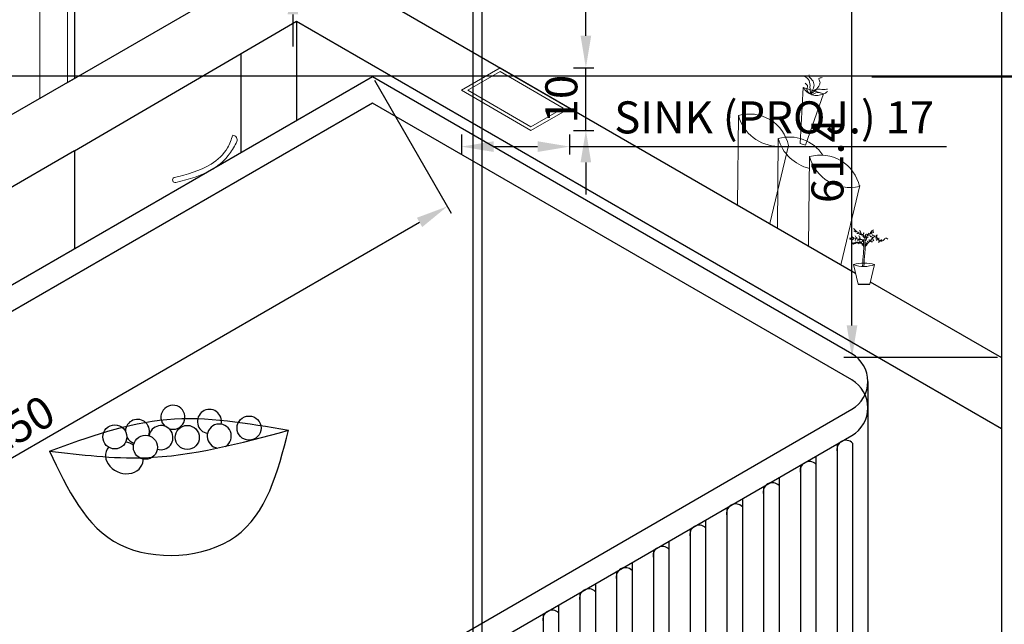
# Model space of a CAD drawing. Units: centimetres. Extents: x 2148 to 2649, y 4226 to 4785.
# Tile 3 of 6: x 2402 to 2555, y 4445 to 4539. Entities that reach past the tile are written whole.
import ezdxf

# ---------------------------------------------------------------- set-up
doc = ezdxf.new("R2010")
doc.units = ezdxf.units.CM
for name, color, linetype, lineweight in [('A-ANNO-DIMS', 63, 'Continuous', 18), ('A-FLOR-BSPL', 21, 'Continuous', 13), ('A-FLOR-CASE', 21, 'Continuous', 25), ('A-FLOR-CASE-HDW', 21, 'Continuous', 18), ('A-FLOR-CASE-TALL', 30, 'Continuous', 30), ('A-FLOR-CTOP', 21, 'Continuous', 25), ('A-FLOR-FIXT', 21, 'Continuous', 18), ('A-FURN-ACCS', 21, 'Continuous', 13), ('TABLE', 30, 'Continuous', 25), ('TREES', 80, 'Continuous', 13)]:
    doc.layers.add(name, color=color, linetype=linetype, lineweight=lineweight)
doc.styles.get("Standard").update_dxf_attribs({"font": 'arial.ttf'})
doc.dimstyles.new('ISO-25', dxfattribs={"dimtxt": 5, "dimasz": 5, "dimexe": 1.25, "dimexo": 0.625, "dimtad": 1, "dimdec": 1, "dimtxsty": 'Standard', "dimcen": 2.5, "dimadec": 0, "dimazin": 0, "dimtfac": 1, "dimtdec": 1, "dimtmove": 0, "dimatfit": 3, "dimfxl": 1, "dimarcsym": 0})

# ---------------------------------------------------------------- blocks, each defined once
blk = doc.blocks.new('RECTANGLE')
for p, q in [((2256.66, 4502.65), (2260.99, 4505.15)), ((2260.99, 4443.76), (2260.99, 4505.15)), ((2256.66, 4502.65), (2256.66, 4441.26)), ((2256.66, 4441.26), (2260.99, 4443.76))]:
    blk.add_line(p, q)
blk = doc.blocks.new('SINK')
for p, q in [((2459.2, 4541.73), (2453.17, 4538.25)), ((2459.2, 4541.73), (2470.05, 4535.47)), ((2459.2, 4541.15), (2454.17, 4538.25)), ((2459.2, 4541.15), (2469.05, 4535.47)), ((2453.17, 4538.25), (2464.01, 4531.98)), ((2454.17, 4538.25), (2464.01, 4532.56)), ((2464.01, 4531.98), (2470.05, 4535.47)), ((2464.01, 4532.56), (2469.05, 4535.47))]:
    blk.add_line(p, q)
blk = doc.blocks.new('TREE')
for p, q in [((2447.25, 4544.96), (2445.48, 4552.43)), ((2451.66, 4544.96), (2453.53, 4552.48))]:
    blk.add_line(p, q)
for centre, radius, start, end in [((2449.6, 4537.88), 15.12, 74.9103, 105.8034), ((2449.44, 4562.68), 11, 248.8663, 291.8473)]:
    blk.add_arc(centre, radius, start, end)
for points, knots in [([(2449.83, 4561.3), (2449.83, 4562.01), (2449.83, 4563.42), (2448.06, 4564.55), (2446.36, 4565.02), (2445.78, 4565.95), (2445.51, 4566.39)], [0, 0, 0, 0, 1.995568, 3.979762, 5.67782, 7.159715, 7.159715, 7.159715, 7.159715]), ([(2445.6, 4565.25), (2445.73, 4565.27), (2445.99, 4565.3), (2446.12, 4564.73), (2446.58, 4565.24), (2446.9, 4564.89), (2447.12, 4564.82), (2447.24, 4564.78)], [0, 0, 0, 0, 0.353698, 0.687974, 1.179754, 1.508828, 1.893119, 1.893119, 1.893119, 1.893119]), ([(2446.1, 4563.4), (2446.2, 4563.04), (2446.31, 4562.66), (2446.75, 4562.63), (2446.69, 4562.48), (2446.67, 4562.4), (2446.66, 4562.35)], [0, 0, 0, 0, 0.953341, 1.006749, 1.098323, 1.293043, 1.293043, 1.293043, 1.293043]), ([(2446.66, 4564.4), (2446.82, 4564.33), (2447.08, 4564.23), (2447.48, 4564.53), (2447.88, 4564.52), (2448.14, 4564.42), (2448.2, 4564.4)], [0, 0, 0, 0, 0.487977, 0.748703, 1.415993, 1.585236, 1.585236, 1.585236, 1.585236]), ([(2447.33, 4563.41), (2447.58, 4563.34), (2447.94, 4563.23), (2447.89, 4562.8), (2447.59, 4562.63), (2448.15, 4562.5), (2448.05, 4562.06), (2448.25, 4562.06), (2448.31, 4562.06)], [0, 0, 0, 0, 0.664801, 0.94436, 1.08206, 1.476917, 1.846316, 2.003009, 2.003009, 2.003009, 2.003009]), ([(2447.76, 4563.97), (2447.97, 4563.94), (2448.19, 4563.91), (2448.52, 4563.93), (2448.62, 4563.77), (2448.92, 4563.75), (2449.11, 4563.68), (2449.26, 4563.62)], [0, 0, 0, 0, 0.637067, 0.675943, 0.960411, 1.092541, 1.560471, 1.560471, 1.560471, 1.560471]), ([(2447.89, 4565.62), (2447.89, 4565.43), (2447.89, 4565.1), (2448.34, 4564.81), (2448.24, 4564.52), (2448.19, 4564.38)], [0, 0, 0, 0, 0.528266, 0.942976, 1.342243, 1.342243, 1.342243, 1.342243]), ([(2448.99, 4563.3), (2449.11, 4563.19), (2449.28, 4563.05), (2449.5, 4562.84), (2449.63, 4562.83), (2449.7, 4562.83)], [0, 0, 0, 0, 0.4862835, 0.6806136, 0.871086, 0.871086, 0.871086, 0.871086]), ([(2449.26, 4563.62), (2449.19, 4563.84), (2449.08, 4564.17), (2449.43, 4564.46), (2449.34, 4564.59), (2449.31, 4564.63)], [0, 0, 0, 0, 0.636403, 0.920765, 1.065556, 1.065556, 1.065556, 1.065556]), ([(2450.14, 4564.1), (2450.1, 4563.96), (2450, 4563.68), (2450.06, 4563.32), (2449.98, 4562.88), (2449.68, 4562.82), (2449.46, 4562.77)], [0, 0, 0, 0, 0.427172, 0.880416, 1.093996, 1.685063, 1.685063, 1.685063, 1.685063]), ([(2449.83, 4561.3), (2450.13, 4561.73), (2450.64, 4562.45), (2450.53, 4563.72), (2451.5, 4564.19), (2452.37, 4564.56), (2452.66, 4565.2), (2452.78, 4565.47)], [0, 0, 0, 0, 1.559218, 2.590263, 3.316916, 4.501885, 5.353772, 5.353772, 5.353772, 5.353772]), ([(2449.98, 4559.44), (2450.53, 4560.09), (2451.61, 4561.35), (2454.23, 4564.3), (2454.67, 4561.58), (2456.89, 4561.05), (2457.55, 4562.97), (2458.29, 4562.41), (2458.61, 4562.17)], [0, 0, 0, 0, 2.950259, 5.736815, 7.202351, 9.196187, 10.495572, 11.481506, 11.481506, 11.481506, 11.481506]), ([(2450.65, 4563.53), (2450.67, 4563.63), (2450.7, 4563.82), (2450.57, 4564.03), (2450.57, 4564.16), (2450.57, 4564.2)], [0, 0, 0, 0, 0.2987758, 0.5629986, 0.6917618, 0.6917618, 0.6917618, 0.6917618]), ([(2450.79, 4563.5), (2450.85, 4563.54), (2451.15, 4563.74), (2451.53, 4563.69), (2451.84, 4563.65)], [0, 0, 0, 0, 0.18742, 1.072841, 1.072841, 1.072841, 1.072841]), ([(2451.14, 4564.01), (2451.19, 4564.03), (2451.33, 4564.07), (2451.2, 4564.29), (2451.26, 4564.44), (2451.3, 4564.5), (2451.32, 4564.51)], [0, 0, 0, 0, 0.131224, 0.3928497, 0.5275017, 0.5966013, 0.5966013, 0.5966013, 0.5966013]), ([(2451.65, 4564.25), (2451.78, 4564.27), (2452.08, 4564.3), (2452.39, 4564.26), (2452.56, 4564.23)], [0, 0, 0, 0, 0.388997, 0.9136239, 0.9136239, 0.9136239, 0.9136239]), ([(2452.65, 4562.49), (2452.63, 4562.64), (2452.59, 4562.93), (2452.3, 4563.47), (2451.98, 4563.24), (2451.82, 4563.12)], [0, 0, 0, 0, 0.45479, 0.92627, 1.425708, 1.425708, 1.425708, 1.425708]), ([(2451.9, 4564.38), (2451.95, 4564.49), (2452.04, 4564.65), (2452.01, 4564.87), (2452.01, 4564.97), (2452.01, 4565)], [0, 0, 0, 0, 0.3358398, 0.5448262, 0.633178, 0.633178, 0.633178, 0.633178]), ([(2452.27, 4564.64), (2452.32, 4564.72), (2452.48, 4564.99), (2452.99, 4564.61), (2453.14, 4564.98), (2453.12, 4565.11), (2453.12, 4565.16)], [0, 0, 0, 0, 0.251714, 0.837833, 1.078551, 1.22335, 1.22335, 1.22335, 1.22335]), ([(2452.4, 4564.8), (2452.41, 4564.88), (2452.43, 4565.06), (2452.32, 4565.32), (2452.44, 4565.42), (2452.47, 4565.45)], [0, 0, 0, 0, 0.2491213, 0.5552893, 0.6860823, 0.6860823, 0.6860823, 0.6860823]), ([(2452.72, 4565.33), (2452.73, 4565.38), (2452.79, 4565.56), (2453.08, 4565.6), (2453.11, 4565.76), (2453.12, 4565.78)], [0, 0, 0, 0, 0.1482784, 0.5567745, 0.6230075, 0.6230075, 0.6230075, 0.6230075]), ([(2453.57, 4563.27), (2453.54, 4563.35), (2453.44, 4563.57), (2453.12, 4563.6), (2452.91, 4563.7), (2452.68, 4563.58), (2452.8, 4563.73), (2452.87, 4563.82)], [0, 0, 0, 0, 0.250514, 0.700182, 0.817059, 0.973893, 1.195588, 1.195588, 1.195588, 1.195588]), ([(2454.21, 4563.26), (2454.25, 4563.33), (2454.32, 4563.45), (2454.32, 4563.75), (2454.55, 4563.67), (2454.65, 4563.66), (2454.69, 4563.66)], [0, 0, 0, 0, 0.2405941, 0.4530054, 0.6562483, 0.7710751, 0.7710751, 0.7710751, 0.7710751]), ([(2449.39, 4560.41), (2449.32, 4560.98), (2449.16, 4562.11), (2447.09, 4562.07), (2445.55, 4562.82), (2444.32, 4562.59), (2443.85, 4562.5)], [0, 0, 0, 0, 1.50196, 2.979977, 5.268293, 6.6547, 6.6547, 6.6547, 6.6547]), ([(2444.83, 4562.66), (2444.5, 4562.55), (2444.06, 4562.4), (2444.1, 4562), (2444.11, 4561.9)], [0, 0, 0, 0, 0.86957, 1.154464, 1.154464, 1.154464, 1.154464]), ([(2444.53, 4563.19), (2444.82, 4563.13), (2445.18, 4563.05), (2445.34, 4562.62), (2445.49, 4562.62), (2445.55, 4562.62)], [0, 0, 0, 0, 0.799643, 1.030684, 1.19755, 1.19755, 1.19755, 1.19755]), ([(2449.45, 4559.33), (2448.92, 4560.14), (2448.1, 4561.4), (2446.22, 4560.44), (2445.17, 4560.51), (2444.56, 4560.54)], [0, 0, 0, 0, 2.40992, 3.739305, 5.578847, 5.578847, 5.578847, 5.578847]), ([(2445.01, 4560.71), (2445.17, 4560.62), (2445.37, 4560.5), (2445.62, 4560.51), (2445.68, 4560.52), (2445.69, 4560.52)], [0, 0, 0, 0, 0.5295015, 0.6942572, 0.7168035, 0.7168035, 0.7168035, 0.7168035]), ([(2445.55, 4562.62), (2445.49, 4562.52), (2445.4, 4562.36), (2445.26, 4562.12), (2445.18, 4561.91), (2445.06, 4561.89), (2445.04, 4561.89)], [0, 0, 0, 0, 0.3536471, 0.5448852, 0.8584322, 0.9118713, 0.9118713, 0.9118713, 0.9118713]), ([(2445.19, 4560.23), (2445.23, 4560.26), (2445.34, 4560.32), (2445.53, 4560.36), (2445.62, 4560.47), (2445.66, 4560.52)], [0, 0, 0, 0, 0.157145, 0.3589113, 0.5662429, 0.5662429, 0.5662429, 0.5662429]), ([(2445.61, 4560.86), (2445.67, 4560.79), (2445.79, 4560.65), (2445.97, 4560.57), (2446.2, 4560.56), (2446.18, 4560.62), (2446.18, 4560.64)], [0, 0, 0, 0, 0.2483933, 0.5604364, 0.6736581, 0.7258462, 0.7258462, 0.7258462, 0.7258462]), ([(2446.61, 4562.36), (2446.46, 4562.28), (2446.22, 4562.17), (2446.12, 4561.86), (2446.12, 4561.72), (2446.13, 4561.68)], [0, 0, 0, 0, 0.4813649, 0.7680471, 0.8975493, 0.8975493, 0.8975493, 0.8975493]), ([(2446.22, 4561.18), (2446.38, 4560.89), (2446.62, 4560.47), (2446.85, 4561.06), (2447.05, 4560.94), (2447.15, 4560.88)], [0, 0, 0, 0, 0.64318, 0.967785, 1.239353, 1.239353, 1.239353, 1.239353]), ([(2448.31, 4562.06), (2448.14, 4561.91), (2447.81, 4561.63), (2447.17, 4562.12), (2447.11, 4561.73), (2447.09, 4561.57)], [0, 0, 0, 0, 0.622646, 1.172708, 1.557766, 1.557766, 1.557766, 1.557766]), ([(2447.66, 4560.97), (2447.54, 4560.94), (2447.32, 4560.88), (2447.34, 4560.55), (2447.21, 4560.45), (2447.15, 4560.41)], [0, 0, 0, 0, 0.333136, 0.6124023, 0.8146283, 0.8146283, 0.8146283, 0.8146283]), ([(2447.69, 4560.54), (2447.73, 4560.56), (2447.88, 4560.64), (2448.15, 4560.5), (2448.26, 4560.67), (2448.31, 4560.74)], [0, 0, 0, 0, 0.1577786, 0.4768013, 0.6980293, 0.6980293, 0.6980293, 0.6980293]), ([(2447.73, 4561.36), (2447.81, 4561.27), (2447.9, 4561.16), (2448.03, 4561), (2448.13, 4560.92), (2448.11, 4560.85), (2448.11, 4560.84)], [0, 0, 0, 0, 0.3534347, 0.4287436, 0.6404395, 0.6555943, 0.6555943, 0.6555943, 0.6555943]), ([(2448.68, 4560.4), (2448.6, 4560.54), (2448.48, 4560.74), (2448.57, 4561.03), (2448.51, 4561.14), (2448.48, 4561.19)], [0, 0, 0, 0, 0.4503193, 0.6632194, 0.8315566, 0.8315566, 0.8315566, 0.8315566]), ([(2448.59, 4560), (2448.64, 4560.01), (2448.72, 4560.02), (2448.85, 4559.94), (2448.99, 4559.99), (2449.05, 4559.93), (2449.05, 4559.93)], [0, 0, 0, 0, 0.1309766, 0.2265734, 0.4607298, 0.4703086, 0.4703086, 0.4703086, 0.4703086]), ([(2449.25, 4561.22), (2449.08, 4561.38), (2448.82, 4561.62), (2448.7, 4561.25), (2448.74, 4561.15), (2448.74, 4561.13)], [0, 0, 0, 0, 0.4936671, 0.7765002, 0.8174683, 0.8174683, 0.8174683, 0.8174683]), ([(2448.91, 4551.67), (2449, 4553.4), (2449.11, 4555.46), (2449.34, 4558.06), (2449.53, 4559.55), (2449.32, 4560.95), (2449.26, 4561.81), (2449.24, 4562.05)], [0, 0, 0, 0, 5.198408, 6.198659, 7.833196, 9.680738, 10.407711, 10.407711, 10.407711, 10.407711]), ([(2449.05, 4559.93), (2449.07, 4560.03), (2449.1, 4560.2), (2449.14, 4560.46), (2449.08, 4560.61), (2449.04, 4560.7)], [0, 0, 0, 0, 0.3315498, 0.4956558, 0.7928621, 0.7928621, 0.7928621, 0.7928621]), ([(2449.44, 4551.69), (2449.53, 4553.42), (2449.64, 4555.48), (2449.87, 4558.08), (2450.05, 4559.57), (2449.85, 4560.97), (2449.78, 4561.83), (2449.77, 4562.07)], [0, 0, 0, 0, 5.198408, 6.198659, 7.833196, 9.680738, 10.407711, 10.407711, 10.407711, 10.407711]), ([(2450.35, 4559.88), (2450.3, 4560.05), (2450.24, 4560.27), (2450.53, 4560.53), (2450.4, 4560.73), (2450.3, 4560.87)], [0, 0, 0, 0, 0.457334, 0.622454, 1.040097, 1.040097, 1.040097, 1.040097]), ([(2450.36, 4562.16), (2450.35, 4562.24), (2450.34, 4562.38), (2450.26, 4562.64), (2450.36, 4562.81), (2450.42, 4562.91)], [0, 0, 0, 0, 0.2419015, 0.4294094, 0.782934, 0.782934, 0.782934, 0.782934]), ([(2450.53, 4562.68), (2450.57, 4562.72), (2450.64, 4562.77), (2450.72, 4562.83), (2450.82, 4562.94), (2451.03, 4562.88), (2451.1, 4563), (2451.12, 4563.03)], [0, 0, 0, 0, 0.1839825, 0.2354423, 0.32084, 0.6015787, 0.715757, 0.715757, 0.715757, 0.715757]), ([(2451.04, 4560.68), (2451.04, 4560.78), (2451.05, 4560.99), (2450.8, 4561.22), (2450.91, 4561.38), (2450.96, 4561.45)], [0, 0, 0, 0, 0.308616, 0.5966018, 0.8330049, 0.8330049, 0.8330049, 0.8330049]), ([(2451.4, 4561.1), (2452.09, 4561.38), (2452.96, 4561.74), (2452.35, 4561.06), (2452.51, 4561), (2452.56, 4560.99)], [0, 0, 0, 0, 1.194027, 1.500255, 1.630788, 1.630788, 1.630788, 1.630788]), ([(2451.48, 4561.19), (2451.51, 4561.32), (2451.55, 4561.5), (2451.46, 4561.77), (2451.47, 4561.92), (2451.48, 4562.03)], [0, 0, 0, 0, 0.3935209, 0.5296667, 0.851575, 0.851575, 0.851575, 0.851575]), ([(2452.32, 4562.14), (2452.6, 4562.23), (2453.1, 4562.38), (2452.98, 4561.72), (2453.18, 4561.6), (2453.24, 4561.57)], [0, 0, 0, 0, 0.657659, 1.152477, 1.342596, 1.342596, 1.342596, 1.342596]), ([(2454.41, 4562.99), (2454.17, 4562.89), (2453.74, 4562.72), (2454.23, 4562.34), (2454.12, 4562.17), (2454.1, 4562.14)], [0, 0, 0, 0, 0.56032, 1.008165, 1.121509, 1.121509, 1.121509, 1.121509]), ([(2454.61, 4562.45), (2454.46, 4562.3), (2454.24, 4562.09), (2454.49, 4561.73), (2454.33, 4561.66), (2454.26, 4561.63)], [0, 0, 0, 0, 0.537826, 0.7745438, 0.9749671, 0.9749671, 0.9749671, 0.9749671]), ([(2455.47, 4561.55), (2455.41, 4561.46), (2455.3, 4561.31), (2455.4, 4560.89), (2455.07, 4560.99), (2454.85, 4561.05)], [0, 0, 0, 0, 0.329722, 0.545126, 1.027082, 1.027082, 1.027082, 1.027082]), ([(2454.99, 4561.88), (2455.08, 4561.98), (2455.24, 4562.14), (2455.11, 4562.39), (2455.18, 4562.62), (2455.26, 4562.61), (2455.28, 4562.61)], [0, 0, 0, 0, 0.3499692, 0.6062162, 0.8045661, 0.8552851, 0.8552851, 0.8552851, 0.8552851]), ([(2455.86, 4561.43), (2455.78, 4561.56), (2455.6, 4561.89), (2456.32, 4561.69), (2456.26, 4561.99), (2456.23, 4562.1)], [0, 0, 0, 0, 0.333961, 0.823844, 1.08993, 1.08993, 1.08993, 1.08993])]:
    blk.add_open_spline(points, degree=3, knots=knots)
blk = doc.blocks.new('T')
for p, q in [((2448.14, 4353.09), (2318.24, 4278.09)), ((2522.91, 4309.92), (2448.14, 4353.09)), ((2403.01, 4232.03), (2522.91, 4301.26))]:
    blk.add_line(p, q)
blk.add_arc((2520.41, 4305.59), 5, 300, 60)
blk = doc.blocks.new('FRUITS')
for centre in [(2437.55, 4475.46), (2416.61, 4474.09), (2427.91, 4474), (2421.39, 4472.47)]:
    blk.add_circle(centre, 1.88)
for centre, start, end in [((2425.68, 4477.15), 250.6785, 228.1131), ((2431.37, 4476.49), 347.1742, 260.6235), ((2420.14, 4474.94), 339.5983, 177.9649), ((2423.8, 4473.97), 252.9307, 170.9248), ((2432.9, 4474.21), 301.9934, 262.6603), ((2420.14, 4474.94), 208.8656, 254.0869)]:
    blk.add_arc(centre, 1.88, start, end)
for start_param, end_param in [(4.471607, 4.914134), (5.976427, 9.8373)]:
    blk.add_ellipse((2418.08, 4470.84), major_axis=(-2.82, 1), ratio=0.809593, start_param=start_param, end_param=end_param)
for points, knots in [([(2406.43, 4471.88), (2412.49, 4474.08), (2424.62, 4478.48), (2437.33, 4476.24), (2443.7, 4475.12)], [0, 0, 0, 0, 18.967698, 37.99902, 37.99902, 37.99902, 37.99902]), ([(2406.43, 4471.88), (2409.22, 4465.94), (2414.78, 4454.12), (2438.7, 4455.69), (2442.02, 4468.59), (2443.7, 4475.12)], [0, 0, 0, 0, 18.249558, 36.298645, 54.808813, 54.808813, 54.808813, 54.808813]), ([(2406.43, 4471.88), (2411.36, 4471.29), (2423.93, 4469.77), (2436.23, 4473.1), (2443.7, 4475.12)], [0, 0, 0, 0, 14.783083, 37.710843, 37.710843, 37.710843, 37.710843])]:
    blk.add_open_spline(points, degree=3, knots=knots)
blk = doc.blocks.new('TABLE 3')
for p, q in [((2534.09, 4482.72), (2534.09, 4425.1)), ((2529.29, 4472.97), (2529.29, 4424.6)), ((2531.69, 4473.13), (2531.69, 4424.8)), ((2531.69, 4473.13), (2531.69, 4424.8)), ((2525.96, 4471.05), (2525.96, 4423.89)), ((2529.29, 4471.74), (2529.29, 4424.6)), ((2523.55, 4469.66), (2523.55, 4424.61)), ((2525.96, 4469.82), (2525.96, 4423.89)), ((2523.55, 4468.43), (2523.55, 4424.61)), ((2520.23, 4467.74), (2520.23, 4430.04)), ((2520.23, 4466.51), (2520.23, 4430.04)), ((2517.82, 4466.35), (2517.82, 4432.4)), ((2517.82, 4465.12), (2517.82, 4432.4)), ((2514.5, 4464.43), (2514.5, 4434.64)), ((2512.09, 4463.04), (2512.09, 4434.39)), ((2512.09, 4461.81), (2512.09, 4434.39)), ((2514.5, 4463.2), (2514.5, 4434.64)), ((2508.76, 4461.12), (2508.76, 4432.32)), ((2506.35, 4459.73), (2506.35, 4430.48)), ((2503.03, 4457.81), (2503.03, 4427.36)), ((2506.35, 4458.5), (2506.35, 4430.48)), ((2500.62, 4456.42), (2500.62, 4424.52)), ((2503.03, 4456.58), (2503.03, 4427.36)), ((2497.3, 4454.5), (2497.3, 4419.33)), ((2500.62, 4455.19), (2500.62, 4424.52)), ((2494.89, 4453.11), (2494.89, 4413.65)), ((2497.3, 4453.27), (2497.3, 4419.33)), ((2491.57, 4451.19), (2491.57, 4413.39)), ((2494.89, 4451.88), (2494.89, 4413.65)), ((2489.16, 4449.8), (2489.16, 4412.9)), ((2491.57, 4449.96), (2491.57, 4413.39)), ((2489.16, 4448.57), (2489.16, 4412.9)), ((2483.42, 4446.49), (2483.42, 4412.26)), ((2485.83, 4447.88), (2485.83, 4412.44)), ((2485.83, 4446.65), (2485.83, 4412.44)), ((2483.42, 4445.26), (2483.42, 4412.26))]:
    blk.add_line(p, q)
for centre in [(2530.67, 4472.12), (2524.94, 4468.81), (2519.2, 4465.5), (2513.47, 4462.19), (2507.74, 4458.88), (2502.01, 4455.57), (2496.27, 4452.26), (2490.54, 4448.95), (2484.81, 4445.64)]:
    blk.add_arc(centre, 1.44, 44.5272, 195.4728)
for name, p in [('T', (8.67, 177.13)), ('T', (8.67, 173.04)), ('FRUITS', (0, 0))]:
    blk.add_blockref(name, p)
blk = doc.blocks.new('PULL-BASE-BOW')
for centre, radius, start, end in [((9.29, 6.64), 0.774, 341.702, 83.222), ((0.41, 0.41), 0.414, 116.0189, 282.6641)]:
    blk.add_arc(centre, radius, start, end)
for points, knots in [([(0.23, 0.79), (2.23, 1.29), (5.42, 2.1), (8.53, 4.9), (9.15, 6.73), (9.38, 7.41)], [0, 0, 0, 0, 6.127515, 9.756066, 11.887711, 11.887711, 11.887711, 11.887711]), ([(0.5, 0.01), (2.55, 0.54), (5.72, 1.35), (8.78, 4.08), (9.68, 5.75), (10.03, 6.4)], [0, 0, 0, 0, 6.234589, 9.67204, 11.894402, 11.894402, 11.894402, 11.894402])]:
    blk.add_open_spline(points, degree=3, knots=knots)
blk = doc.blocks.new('*D28')
at = {"layer": 'A-ANNO-DIMS', "color": 0, "lineweight": -2, "transparency": 16777216}
for p, q in [((2470.68, 4521.25), (2470.68, 4518.09)), ((2487.56, 4521.25), (2487.56, 4518.09)), ((2475.68, 4519.34), (2482.56, 4519.34)), ((2487.56, 4519.34), (2546.35, 4519.34))]:
    blk.add_line(p, q, dxfattribs=at)
at = {"layer": 'A-ANNO-DIMS', "color": 0, "transparency": 16777216}
for points in [[(2475.68, 4520.17), (2475.68, 4518.51), (2470.68, 4519.34)], [(2482.56, 4520.17), (2482.56, 4518.51), (2487.56, 4519.34)]]:
    blk.add_solid(points, dxfattribs=at)
at = {"layer": 'Defpoints', "color": 0, "transparency": 16777216}
for p in [(2470.68, 4521.87), (2487.56, 4521.87), (2487.56, 4519.34)]:
    blk.add_point(p, dxfattribs=at)
at = {"layer": 'A-ANNO-DIMS', "color": 0, "transparency": 16777216, "insert": (2519.46, 4523.25), "char_height": 5, "attachment_point": 5}
blk.add_mtext('SINK (PROJ.) 17', dxfattribs=at)
blk = doc.blocks.new('*D29')
at = {"layer": 'A-ANNO-DIMS', "color": 0, "lineweight": -2, "transparency": 16777216}
for p, q in [((2490.09, 4536.62), (2490.09, 4541.62)), ((2488.18, 4531.62), (2491.34, 4531.62)), ((2490.09, 4521.87), (2490.09, 4531.62)), ((2488.18, 4521.87), (2491.34, 4521.87)), ((2490.09, 4516.87), (2490.09, 4511.87))]:
    blk.add_line(p, q, dxfattribs=at)
at = {"layer": 'A-ANNO-DIMS', "color": 0, "transparency": 16777216}
for points in [[(2489.26, 4536.62), (2490.92, 4536.62), (2490.09, 4531.62)], [(2489.26, 4516.87), (2490.92, 4516.87), (2490.09, 4521.87)]]:
    blk.add_solid(points, dxfattribs=at)
at = {"layer": 'Defpoints', "color": 0, "transparency": 16777216}
for p in [(2487.56, 4531.62), (2490.09, 4531.62), (2487.56, 4521.87)]:
    blk.add_point(p, dxfattribs=at)
at = {"layer": 'A-ANNO-DIMS', "color": 0, "transparency": 16777216, "insert": (2486.91, 4526.75), "char_height": 5, "attachment_point": 5, "rotation": 90}
blk.add_mtext('10', dxfattribs=at)
blk = doc.blocks.new('*D30')
at = {"layer": 'A-ANNO-DIMS', "color": 0, "lineweight": -2, "transparency": 16777216}
for p, q in [((2534.71, 4530.22), (2574.8, 4530.22)), ((2573.55, 4272.15), (2573.55, 4525.22)), ((2534.71, 4267.15), (2574.8, 4267.15))]:
    blk.add_line(p, q, dxfattribs=at)
at = {"layer": 'A-ANNO-DIMS', "color": 0, "transparency": 16777216}
for points in [[(2572.71, 4525.22), (2574.38, 4525.22), (2573.55, 4530.22)], [(2572.71, 4272.15), (2574.38, 4272.15), (2573.55, 4267.15)]]:
    blk.add_solid(points, dxfattribs=at)
at = {"layer": 'Defpoints', "color": 0, "transparency": 16777216}
for p in [(2534.09, 4530.22), (2573.55, 4530.22), (2534.09, 4267.15)]:
    blk.add_point(p, dxfattribs=at)
at = {"layer": 'A-ANNO-DIMS', "color": 0, "transparency": 16777216, "insert": (2569.64, 4398.69), "char_height": 5, "attachment_point": 5, "rotation": 90}
blk.add_mtext('ISLAND (PROJ.) 263', dxfattribs=at)
blk = doc.blocks.new('*D38')
at = {"layer": 'A-ANNO-DIMS', "color": 0, "lineweight": -2, "transparency": 16777216}
for p, q in [((2444.39, 4558.67), (2444.39, 4609.58)), ((2443.71, 4553.67), (2445.64, 4553.67)), ((2444.39, 4544.96), (2444.39, 4553.67)), ((2443.71, 4544.96), (2445.64, 4544.96)), ((2444.39, 4539.96), (2444.39, 4534.96))]:
    blk.add_line(p, q, dxfattribs=at)
at = {"layer": 'A-ANNO-DIMS', "color": 0, "transparency": 16777216}
for points in [[(2443.56, 4558.67), (2445.22, 4558.67), (2444.39, 4553.67)], [(2443.56, 4539.96), (2445.22, 4539.96), (2444.39, 4544.96)]]:
    blk.add_solid(points, dxfattribs=at)
at = {"layer": 'Defpoints', "color": 0, "transparency": 16777216}
for p in [(2443.09, 4553.67), (2444.39, 4553.67), (2443.09, 4544.96)]:
    blk.add_point(p, dxfattribs=at)
at = {"layer": 'A-ANNO-DIMS', "color": 0, "transparency": 16777216, "insert": (2441.21, 4586.62), "char_height": 5, "attachment_point": 5, "rotation": 90}
blk.add_mtext('PLANT 9 TYP.', dxfattribs=at)
blk = doc.blocks.new('*D44')
at = {"layer": 'A-ANNO-DIMS', "color": 0, "lineweight": -2, "transparency": 16777216}
for p, q in [((2305.27, 4564.32), (2648.78, 4564.32)), ((2647.53, 4559.32), (2647.53, 4535.36)), ((2305.27, 4530.36), (2648.78, 4530.36))]:
    blk.add_line(p, q, dxfattribs=at)
at = {"layer": 'A-ANNO-DIMS', "color": 0, "transparency": 16777216}
for points in [[(2646.7, 4559.32), (2648.37, 4559.32), (2647.53, 4564.32)], [(2646.7, 4535.36), (2648.37, 4535.36), (2647.53, 4530.36)]]:
    blk.add_solid(points, dxfattribs=at)
at = {"layer": 'Defpoints', "color": 0, "transparency": 16777216}
for p in [(2304.65, 4564.32), (2304.65, 4530.36), (2647.53, 4530.36)]:
    blk.add_point(p, dxfattribs=at)
at = {"layer": 'A-ANNO-DIMS', "color": 0, "transparency": 16777216, "insert": (2644.35, 4547.34), "char_height": 5, "attachment_point": 5, "rotation": 90}
blk.add_mtext('33.96', dxfattribs=at)
blk = doc.blocks.new('*D48')
at = {"layer": 'A-ANNO-DIMS', "color": 0, "lineweight": -2, "transparency": 16777216}
for p, q in [((2472.44, 4594.86), (2472.44, 4242.8)), ((2473.86, 4594.94), (2473.86, 4242.8)), ((2467.44, 4244.05), (2462.44, 4244.05)), ((2472.44, 4244.05), (2473.86, 4244.05)), ((2478.86, 4244.05), (2497.57, 4244.05))]:
    blk.add_line(p, q, dxfattribs=at)
at = {"layer": 'A-ANNO-DIMS', "color": 0, "transparency": 16777216}
for points in [[(2467.44, 4244.88), (2467.44, 4243.21), (2472.44, 4244.05)], [(2478.86, 4244.88), (2478.86, 4243.21), (2473.86, 4244.05)]]:
    blk.add_solid(points, dxfattribs=at)
at = {"layer": 'Defpoints', "color": 0, "transparency": 16777216}
for p in [(2472.44, 4595.48), (2473.86, 4595.56), (2473.86, 4244.05)]:
    blk.add_point(p, dxfattribs=at)
at = {"layer": 'A-ANNO-DIMS', "color": 0, "transparency": 16777216, "insert": (2490.71, 4247.18), "char_height": 5, "attachment_point": 5}
blk.add_mtext('1.42', dxfattribs=at)
blk = doc.blocks.new('*D51')
at = {"layer": 'A-ANNO-DIMS', "color": 0, "lineweight": -2, "transparency": 16777216}
for p, q in [((2436.91, 4714.24), (2648.78, 4714.24)), ((2647.53, 4272.37), (2647.53, 4709.24)), ((2409.81, 4267.37), (2648.78, 4267.37))]:
    blk.add_line(p, q, dxfattribs=at)
at = {"layer": 'A-ANNO-DIMS', "color": 0, "transparency": 16777216}
for points in [[(2646.7, 4709.24), (2648.37, 4709.24), (2647.53, 4714.24)], [(2646.7, 4272.37), (2648.37, 4272.37), (2647.53, 4267.37)]]:
    blk.add_solid(points, dxfattribs=at)
at = {"layer": 'Defpoints', "color": 0, "transparency": 16777216}
for p in [(2436.28, 4714.24), (2647.53, 4714.24), (2409.18, 4267.37)]:
    blk.add_point(p, dxfattribs=at)
at = {"layer": 'A-ANNO-DIMS', "color": 0, "transparency": 16777216, "insert": (2644.36, 4490.81), "char_height": 5, "attachment_point": 5, "rotation": 90}
blk.add_mtext('446.9', dxfattribs=at)
blk = doc.blocks.new('*D58')
at = {"layer": 'A-ANNO-DIMS', "color": 0, "lineweight": -2, "transparency": 16777216}
for p, q in [((2457.13, 4529.68), (2469.1, 4508.94)), ((2464.15, 4507.52), (2342.9, 4437.52)), ((2327.22, 4454.68), (2339.2, 4433.94))]:
    blk.add_line(p, q, dxfattribs=at)
at = {"layer": 'A-ANNO-DIMS', "color": 0, "transparency": 16777216}
for points in [[(2463.73, 4508.25), (2464.56, 4506.8), (2468.48, 4510.02)], [(2342.49, 4438.25), (2343.32, 4436.8), (2338.57, 4435.02)]]:
    blk.add_solid(points, dxfattribs=at)
at = {"layer": 'Defpoints', "color": 0, "transparency": 16777216}
for p in [(2456.81, 4530.22), (2326.91, 4455.22), (2338.57, 4435.02)]:
    blk.add_point(p, dxfattribs=at)
at = {"layer": 'A-ANNO-DIMS', "color": 0, "transparency": 16777216, "insert": (2401.94, 4475.28), "char_height": 5, "attachment_point": 5, "rotation": 30}
blk.add_mtext('150', dxfattribs=at)
blk = doc.blocks.new('*D59')
at = {"layer": 'A-ANNO-DIMS', "color": 0, "lineweight": -2, "transparency": 16777216}
for p, q in [((2554.3, 4547.86), (2530.35, 4547.86)), ((2531.6, 4491.46), (2531.6, 4542.86)), ((2554.3, 4486.46), (2530.35, 4486.46))]:
    blk.add_line(p, q, dxfattribs=at)
at = {"layer": 'A-ANNO-DIMS', "color": 0, "transparency": 16777216}
for points in [[(2530.77, 4542.86), (2532.43, 4542.86), (2531.6, 4547.86)], [(2530.77, 4491.46), (2532.43, 4491.46), (2531.6, 4486.46)]]:
    blk.add_solid(points, dxfattribs=at)
at = {"layer": 'Defpoints', "color": 0, "transparency": 16777216}
for p in [(2531.6, 4547.86), (2554.93, 4547.86), (2554.93, 4486.46)]:
    blk.add_point(p, dxfattribs=at)
at = {"layer": 'A-ANNO-DIMS', "color": 0, "transparency": 16777216, "insert": (2528.42, 4517.16), "char_height": 5, "attachment_point": 5, "rotation": 90}
blk.add_mtext('61.4', dxfattribs=at)

msp = doc.modelspace()

# ---------------------------------------------------------------- linework, layer by layer
at = {"layer": 'A-FLOR-CASE'}
for p, q in [((2410.3004, 4699.2447), (2410.3004, 4529.9623)), ((2444.9414, 4538.8707), (2444.9414, 4523.3687)), ((2436.2812, 4533.8172), (2436.2812, 4518.3687)), ((2410.3004, 4518.6569), (2410.3004, 4503.3687))]:
    msp.add_line(p, q, dxfattribs=at)
at = {"layer": 'A-FLOR-CASE-TALL'}
msp.add_line((2554.9266, 4645.7447), (2554.9266, 4369.7671), dxfattribs=at)
at = {"layer": 'A-FLOR-CTOP'}
for p, q in [((2409.2302, 4529.3444), (2436.2812, 4544.9623)), ((2453.6017, 4544.9623), (2532.1733, 4499.5989)), ((2410.3004, 4518.6569), (2444.9414, 4538.8707)), ((2444.9414, 4538.8707), (2554.9266, 4475.3707)), ((2410.3004, 4529.9623), (2254.4158, 4439.9623)), ((2410.3004, 4518.6569), (2254.4158, 4428.6569)), ((2532.5706, 4497.9209), (2534.3632, 4497.9209)), ((2534.4534, 4498.2825), (2554.9266, 4486.4623))]:
    msp.add_line(p, q, dxfattribs=at)
at = {"layer": 'A-FURN-ACCS'}
for p, q in [((2513.7427, 4510.2398), (2513.8843, 4524.1808)), ((2519.9592, 4506.6507), (2520.1007, 4520.5917)), ((2521.6845, 4519.5131), (2518.7703, 4507.3371)), ((2524.8302, 4503.8385), (2524.9717, 4517.7794)), ((2532.8065, 4513.256), (2529.8577, 4500.9358)), ((2513.7427, 4510.2398), (2518.7703, 4507.3371)), ((2519.9592, 4506.6507), (2524.9867, 4503.7481)), ((2524.8302, 4503.8385), (2529.8577, 4500.9358))]:
    msp.add_line(p, q, dxfattribs=at)
for centre, radius, start, end in [((2515.6078, 4518.2096), 6.2149, 12.106803, 106.100627), ((2520.2607, 4525.9851), 6.6267, 195.799765, 268.508977), ((2521.8243, 4514.6206), 6.2149, 33.095394, 106.100627), ((2526.4771, 4522.396), 6.6267, 195.799765, 256.704649), ((2526.6953, 4511.8083), 6.2149, 12.106803, 106.100627), ((2531.3481, 4519.5837), 6.6267, 195.799765, 282.407665)]:
    msp.add_arc(centre, radius, start, end, dxfattribs=at)
at = {"layer": 'TABLE'}
msp.add_line((2508.7637, 4459.8889), (2508.7637, 4432.3196), dxfattribs=at)
at = {"layer": 'TREES'}
for p, q in [((2523.5086, 4519.8148), (2524.0096, 4528.579)), ((2524.0096, 4528.579), (2527.1342, 4527.5826)), ((2527.1342, 4527.5826), (2524.3631, 4519.5409)), ((2524.3631, 4519.5409), (2523.5086, 4519.8148))]:
    msp.add_line(p, q, dxfattribs=at)
msp.add_arc((2526.0501, 4529.5804), 2.273, 206.140299, 298.485133, dxfattribs=at)
for points, knots in [([(2525.1443, 4527.5393), (2525.0928, 4527.8926), (2525.0162, 4528.4173), (2525.0929, 4529.2921), (2524.7724, 4529.9979), (2524.3149, 4530.2026), (2524.1847, 4530.2608)], [0, 0, 0, 0, 1.06374187, 1.57967804, 2.64384145, 3.06726213, 3.06726213, 3.06726213, 3.06726213]), ([(2525.1256, 4527.504), (2525.4714, 4528.156), (2525.9808, 4529.1162), (2525.2201, 4529.9182), (2524.835, 4530.2969), (2524.8871, 4530.4701), (2524.9017, 4530.5188)], [0, 0, 0, 0, 1.90458252, 2.80483992, 3.17863294, 3.32478922, 3.32478922, 3.32478922, 3.32478922]), ([(2525.1256, 4527.504), (2525.7075, 4527.928), (2526.4295, 4528.4542), (2526.6803, 4529.456), (2526.26, 4530.0772), (2526.7322, 4530.085), (2526.9668, 4530.0889)], [0, 0, 0, 0, 2.03544398, 2.52608335, 3.06157979, 3.59043119, 3.59043119, 3.59043119, 3.59043119]), ([(2525.3596, 4527.4149), (2524.9162, 4527.6673), (2524.4295, 4527.9444), (2524.6329, 4528.5027), (2524.7362, 4528.8223), (2524.4713, 4529.0521), (2524.3551, 4529.1716), (2524.2994, 4529.229)], [0, 0, 0, 0, 1.18190811, 1.29741505, 1.76342462, 2.02775855, 2.27105241, 2.27105241, 2.27105241, 2.27105241]), ([(2525.3596, 4527.4149), (2525.7475, 4527.6446), (2526.3364, 4527.9933), (2527.1773, 4527.4243), (2527.5634, 4527.7597), (2527.7699, 4527.9391)], [0, 0, 0, 0, 1.22473141, 1.85882723, 2.58769727, 2.58769727, 2.58769727, 2.58769727]), ([(2525.5719, 4528.0808), (2525.7291, 4528.15), (2526.2415, 4528.3753), (2526.9613, 4528.2068), (2527.5399, 4528.2868), (2527.7412, 4528.2839), (2527.7986, 4528.2831)], [0, 0, 0, 0, 0.50769505, 1.65497128, 2.08615363, 2.25824683, 2.25824683, 2.25824683, 2.25824683])]:
    msp.add_open_spline(points, degree=3, knots=knots, dxfattribs=at)

# ---------------------------------------------------------------- block references
at = {"layer": 'A-FLOR-BSPL'}
msp.add_blockref('RECTANGLE', (148.243, 85.5881), dxfattribs=at)
at = {"layer": 'A-FLOR-CASE-HDW'}
msp.add_blockref('PULL-BASE-BOW', (2425.6302, 4513.7245), dxfattribs=at)
at = {"layer": 'A-FLOR-FIXT'}
msp.add_blockref('SINK', (17.5116, -10.1103), dxfattribs=at)
at = {"layer": 'TABLE'}
msp.add_blockref('TABLE 3', (0, 0), dxfattribs=at)
at = {"layer": 'TREES', "xscale": 0.4062539037300824, "yscale": 0.4062539037300824, "zscale": 0.4062539037300824}
msp.add_blockref('TREE', (1538.3674, 2651.5123), dxfattribs=at)

# ---------------------------------------------------------------- dimensions: what is measured, and where the dimension line sits
at = {"layer": 'A-ANNO-DIMS'}
for base, p1, p2, angle, override, picture, middle in [((2647.5337, 4714.2447), (2409.1829, 4267.3731), (2436.2812, 4714.2447), 90, {"dimdec": 1, "dimlfac": 1, "dimrnd": 0, "dimzin": 0, "dimdsep": 46, "dimlunit": 2}, '*D51', (2644.3558, 4490.8089)), ((2647.5337, 4530.357), (2304.6453, 4564.3196), (2304.6453, 4530.357), 90, {"dimdec": 2, "dimlfac": 1, "dimrnd": 0, "dimzin": 0, "dimdsep": 46, "dimlunit": 2}, '*D44', (2644.3541, 4547.3383)), ((2531.6016, 4547.857), (2554.9266, 4486.4623), (2554.9266, 4547.857), 90, {"dimdec": 1, "dimlfac": 1, "dimrnd": 0, "dimzin": 0, "dimdsep": 46, "dimlunit": 2}, '*D59', (2528.4238, 4517.1596)), ((2490.0907, 4531.6197), (2487.5585, 4521.8734), (2487.5585, 4531.6197), 90, {"dimdec": 0, "dimlfac": 1, "dimrnd": 0, "dimzin": 0, "dimdsep": 46, "dimlunit": 2}, '*D29', (2486.9129, 4526.7466)), ((2338.573, 4435.0235), (2456.8143, 4530.2236), (2326.9105, 4455.2236), 210, {"dimdec": 0, "dimlfac": 1, "dimrnd": 0, "dimzin": 0, "dimdsep": 46, "dimlunit": 2}, '*D58', (2401.936, 4475.2756))]:
    dim = msp.add_linear_dim(base=base, p1=p1, p2=p2, angle=angle, dimstyle='ISO-25', override=override, dxfattribs=at)
    dim.commit()
    dim.dimension.update_dxf_attribs({"geometry": picture, "text_midpoint": middle})
for base, p1, p2, text, picture, middle in [((2444.391, 4553.6666), (2443.0854, 4544.9623), (2443.0854, 4553.6666), 'PLANT <> TYP.', '*D38', (2441.2132, 4586.621)), ((2573.5478, 4530.2236), (2534.0868, 4267.1498), (2534.0868, 4530.2236), 'ISLAND (PROJ.) <>', '*D30', (2569.6435, 4398.6867))]:
    dim = msp.add_linear_dim(base=base, p1=p1, p2=p2, angle=90, text=text, dimstyle='ISO-25', override={"dimdec": 0, "dimlfac": 1, "dimrnd": 0, "dimzin": 0, "dimdsep": 46, "dimlunit": 2}, dxfattribs=at)
    dim.commit()
    dim.dimension.update_dxf_attribs({"geometry": picture, "text_midpoint": middle})
dim = msp.add_linear_dim(base=(2473.8561, 4244.0481), p1=(2472.4377, 4595.482), p2=(2473.8561, 4595.5637), dimstyle='ISO-25', override={"dimdec": 2, "dimlfac": 1, "dimrnd": 0, "dimzin": 0, "dimdsep": 46, "dimlunit": 2}, dxfattribs=at)
dim.commit()
dim.dimension.update_dxf_attribs({"geometry": '*D48', "text_midpoint": (2490.714, 4247.1833)})
dim = msp.add_linear_dim(base=(2487.5585, 4519.3412), p1=(2470.6773, 4521.8734), p2=(2487.5585, 4521.8734), text='SINK (PROJ.) <>', dimstyle='ISO-25', override={"dimdec": 0, "dimlfac": 1, "dimrnd": 0, "dimzin": 0, "dimdsep": 46, "dimlunit": 2}, dxfattribs=at)
dim.commit()
dim.dimension.update_dxf_attribs({"geometry": '*D28', "text_midpoint": (2519.4557, 4523.2455)})

doc.saveas('drawing.dxf')
